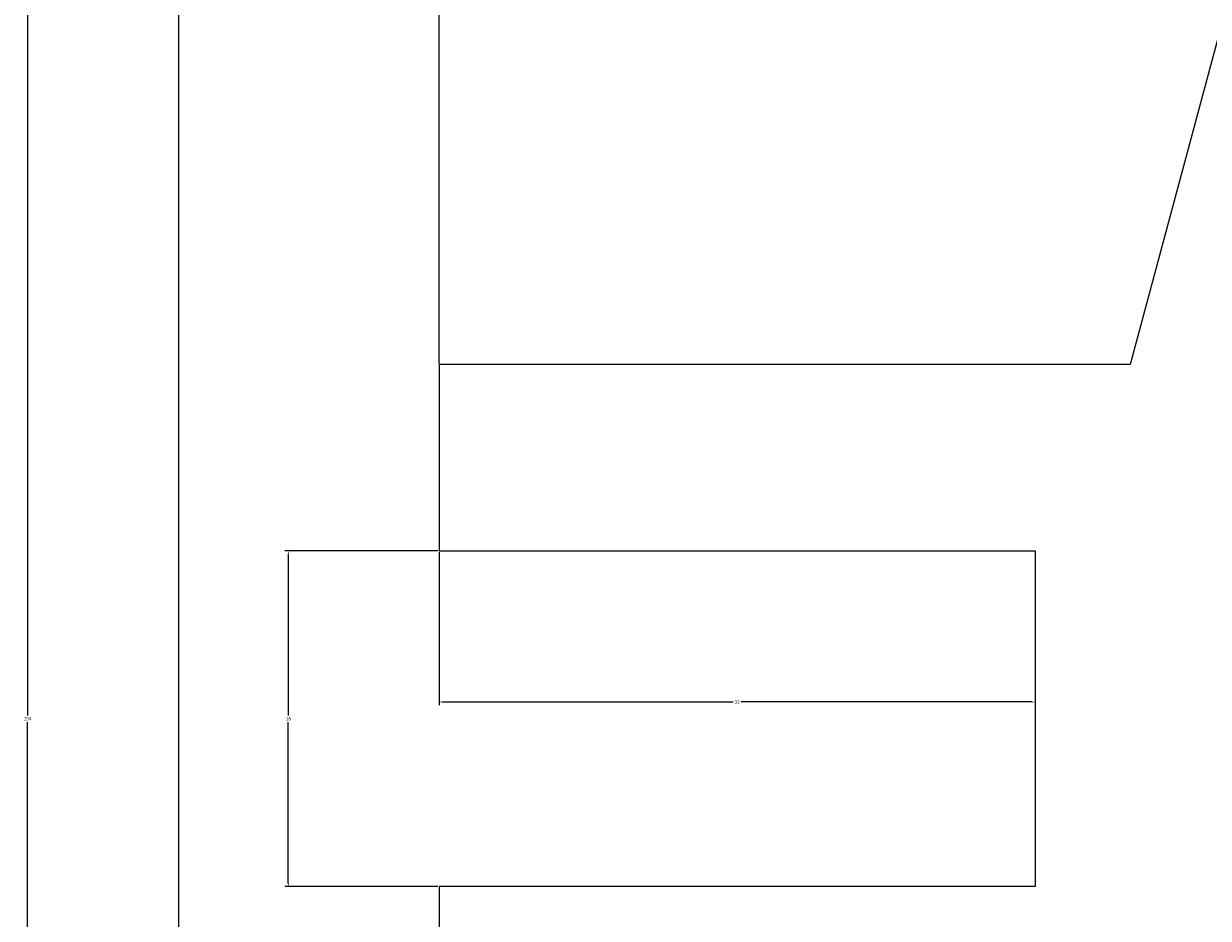
# Model space of a CAD drawing. Units: millimetres. Extents: x 2597 to 2768, y 1809 to 1980.
# Tile 2 of 7: x 2597 to 2661, y 1884 to 1932. Entities that reach past the tile are written whole.
import ezdxf

# ---------------------------------------------------------------- set-up
doc = ezdxf.new("R2010")
doc.units = ezdxf.units.MM
doc.layers.add('M-CONS', color=8, linetype='Continuous', lineweight=18)
doc.layers.add('M-DIMS', color=2, linetype='Continuous', lineweight=18)
doc.styles.get("Standard").update_dxf_attribs({"font": 'arial.ttf'})
doc.dimstyles.get("Standard").update_dxf_attribs({"dimtxt": 0.18, "dimasz": 0.18, "dimexe": 0.18, "dimexo": 0.0625, "dimgap": 0.09, "dimtad": 0, "dimtih": 1, "dimtoh": 1, "dimdec": 4, "dimzin": 0, "dimdsep": 46, "dimtxsty": 'Standard', "dimcen": 0.09, "dimadec": 0, "dimazin": 0, "dimtfac": 1, "dimtdec": 4, "dimtofl": 0, "dimtmove": 0, "dimatfit": 3, "dimfxl": 1, "dimtolj": 1, "dimtzin": 0, "dimarcsym": 0})

# ---------------------------------------------------------------- blocks, each defined once
blk = doc.blocks.new('*D4')
at = {"layer": 'Defpoints', "color": 0, "transparency": 16777216}
for p in [(2597.676, 1971.43), (2631.776, 1971.43), (2631.776, 1817.43)]:
    blk.add_point(p, dxfattribs=at)
at = {"layer": 'M-DIMS', "color": 0, "lineweight": -2, "transparency": 16777216}
for p, q in [((2631.713, 1971.43), (2597.496, 1971.43)), ((2597.676, 1971.25), (2597.676, 1894.612)), ((2597.676, 1817.61), (2597.676, 1894.248)), ((2631.713, 1817.43), (2597.496, 1817.43))]:
    blk.add_line(p, q, dxfattribs=at)
at = {"layer": 'M-DIMS', "color": 0, "transparency": 16777216}
for points in [[(2597.646, 1971.25), (2597.706, 1971.25), (2597.676, 1971.43)], [(2597.646, 1817.61), (2597.706, 1817.61), (2597.676, 1817.43)]]:
    blk.add_solid(points, dxfattribs=at)
at = {"layer": 'M-DIMS', "color": 0, "transparency": 16777216, "insert": (2597.676, 1894.43), "char_height": 0.18, "attachment_point": 5}
blk.add_mtext('\\A1;154', dxfattribs=at)
blk = doc.blocks.new('*D8')
at = {"layer": 'Defpoints', "color": 0, "transparency": 16777216}
for p in [(2619.776, 1979.53), (2605.776, 1945.43), (2619.776, 1913.43)]:
    blk.add_point(p, dxfattribs=at)
at = {"layer": 'M-DIMS', "color": 0, "lineweight": -2, "transparency": 16777216}
for p, q in [((2605.776, 1945.493), (2605.776, 1979.71)), ((2605.956, 1979.53), (2612.565, 1979.53)), ((2619.596, 1979.53), (2612.986, 1979.53)), ((2619.776, 1913.493), (2619.776, 1979.71))]:
    blk.add_line(p, q, dxfattribs=at)
at = {"layer": 'M-DIMS', "color": 0, "transparency": 16777216}
for points in [[(2605.956, 1979.56), (2605.956, 1979.5), (2605.776, 1979.53)], [(2619.596, 1979.56), (2619.596, 1979.5), (2619.776, 1979.53)]]:
    blk.add_solid(points, dxfattribs=at)
at = {"layer": 'M-DIMS', "color": 0, "transparency": 16777216, "insert": (2612.776, 1979.53), "char_height": 0.18, "attachment_point": 5}
blk.add_mtext('\\A1;14', dxfattribs=at)
blk = doc.blocks.new('*D9')
at = {"layer": 'Defpoints', "color": 0, "transparency": 16777216}
for p in [(2619.776, 1903.43), (2651.776, 1903.43), (2619.776, 1895.33)]:
    blk.add_point(p, dxfattribs=at)
at = {"layer": 'M-DIMS', "color": 0, "lineweight": -2, "transparency": 16777216}
for p, q in [((2619.776, 1903.368), (2619.776, 1895.15)), ((2651.776, 1903.368), (2651.776, 1895.15)), ((2619.956, 1895.33), (2635.558, 1895.33)), ((2651.596, 1895.33), (2635.994, 1895.33))]:
    blk.add_line(p, q, dxfattribs=at)
at = {"layer": 'M-DIMS', "color": 0, "transparency": 16777216}
for points in [[(2619.956, 1895.36), (2619.956, 1895.3), (2619.776, 1895.33)], [(2651.596, 1895.36), (2651.596, 1895.3), (2651.776, 1895.33)]]:
    blk.add_solid(points, dxfattribs=at)
at = {"layer": 'M-DIMS', "color": 0, "transparency": 16777216, "insert": (2635.776, 1895.33), "char_height": 0.18, "attachment_point": 5}
blk.add_mtext('\\A1;32', dxfattribs=at)
blk = doc.blocks.new('*D10')
at = {"layer": 'Defpoints', "color": 0, "transparency": 16777216}
for p in [(2611.676, 1903.43), (2619.776, 1903.43), (2619.776, 1885.43)]:
    blk.add_point(p, dxfattribs=at)
at = {"layer": 'M-DIMS', "color": 0, "lineweight": -2, "transparency": 16777216}
for p, q in [((2619.713, 1903.43), (2611.496, 1903.43)), ((2611.676, 1903.25), (2611.676, 1894.612)), ((2611.676, 1885.61), (2611.676, 1894.248)), ((2619.713, 1885.43), (2611.496, 1885.43))]:
    blk.add_line(p, q, dxfattribs=at)
at = {"layer": 'M-DIMS', "color": 0, "transparency": 16777216}
for points in [[(2611.646, 1903.25), (2611.706, 1903.25), (2611.676, 1903.43)], [(2611.646, 1885.61), (2611.706, 1885.61), (2611.676, 1885.43)]]:
    blk.add_solid(points, dxfattribs=at)
at = {"layer": 'M-DIMS', "color": 0, "transparency": 16777216, "insert": (2611.676, 1894.43), "char_height": 0.18, "attachment_point": 5}
blk.add_mtext('\\A1;18', dxfattribs=at)

msp = doc.modelspace()

# ---------------------------------------------------------------- linework, layer by layer
at = {"layer": 'M-CONS'}
msp.add_lwpolyline([(2631.7756, 1817.4301), (2733.7756, 1817.4301, 0.4142136), (2759.7756, 1843.4301), (2759.7756, 1945.4301, 0.4142136), (2733.7756, 1971.4301), (2631.7756, 1971.4301, 0.4142136), (2605.7756, 1945.4301), (2605.7756, 1843.4301, 0.4142136)], format="xyb", close=True, dxfattribs=at)
msp.add_lwpolyline([(2713.7756, 1903.4301), (2745.7756, 1903.4301), (2745.7756, 1913.4301), (2708.6698, 1913.4301), (2700.1588, 1945.1014, 0.7667514), (2665.3923, 1945.1014), (2656.8814, 1913.4301), (2619.7756, 1913.4301), (2619.7756, 1903.4301), (2651.7756, 1903.4301), (2651.7756, 1885.4301), (2619.7756, 1885.4301), (2619.7756, 1875.4301), (2656.8814, 1875.4301), (2665.3923, 1843.7587, 0.7667514), (2700.1588, 1843.7587), (2708.6698, 1875.4301), (2745.7756, 1875.4301), (2745.7756, 1885.4301), (2713.7756, 1885.4301), (2713.7756, 1903.4301), (2713.7756, 1894.4301)], format="xyb", dxfattribs=at)

# ---------------------------------------------------------------- dimensions: what is measured, and where the dimension line sits
at = {"layer": 'M-DIMS'}
dim = msp.add_linear_dim(base=(2619.7756, 1979.5301), p1=(2605.7756, 1945.4301), p2=(2619.7756, 1913.4301), dimstyle='Standard', override={"dimdec": 0, "dimlfac": 1, "dimrnd": 0, "dimzin": 0, "dimdsep": 46, "dimlunit": 2}, dxfattribs=at)
dim.commit()
dim.dimension.update_dxf_attribs({"geometry": '*D8', "text_midpoint": (2612.7756, 1979.5301)})
for base, p1, p2, angle, picture, middle in [((2597.6756, 1971.4301), (2631.7756, 1817.4301), (2631.7756, 1971.4301), 90, '*D4', (2597.6756, 1894.4301)), ((2611.6756, 1903.4301), (2619.7756, 1885.4301), (2619.7756, 1903.4301), 90, '*D10', (2611.6756, 1894.4301)), ((2619.7756, 1895.3301), (2651.7756, 1903.4301), (2619.7756, 1903.4301), 180, '*D9', (2635.7756, 1895.3301))]:
    dim = msp.add_linear_dim(base=base, p1=p1, p2=p2, angle=angle, dimstyle='Standard', override={"dimdec": 0, "dimlfac": 1, "dimrnd": 0, "dimzin": 0, "dimdsep": 46, "dimlunit": 2}, dxfattribs=at)
    dim.commit()
    dim.dimension.update_dxf_attribs({"geometry": picture, "text_midpoint": middle})

doc.saveas('drawing.dxf')
